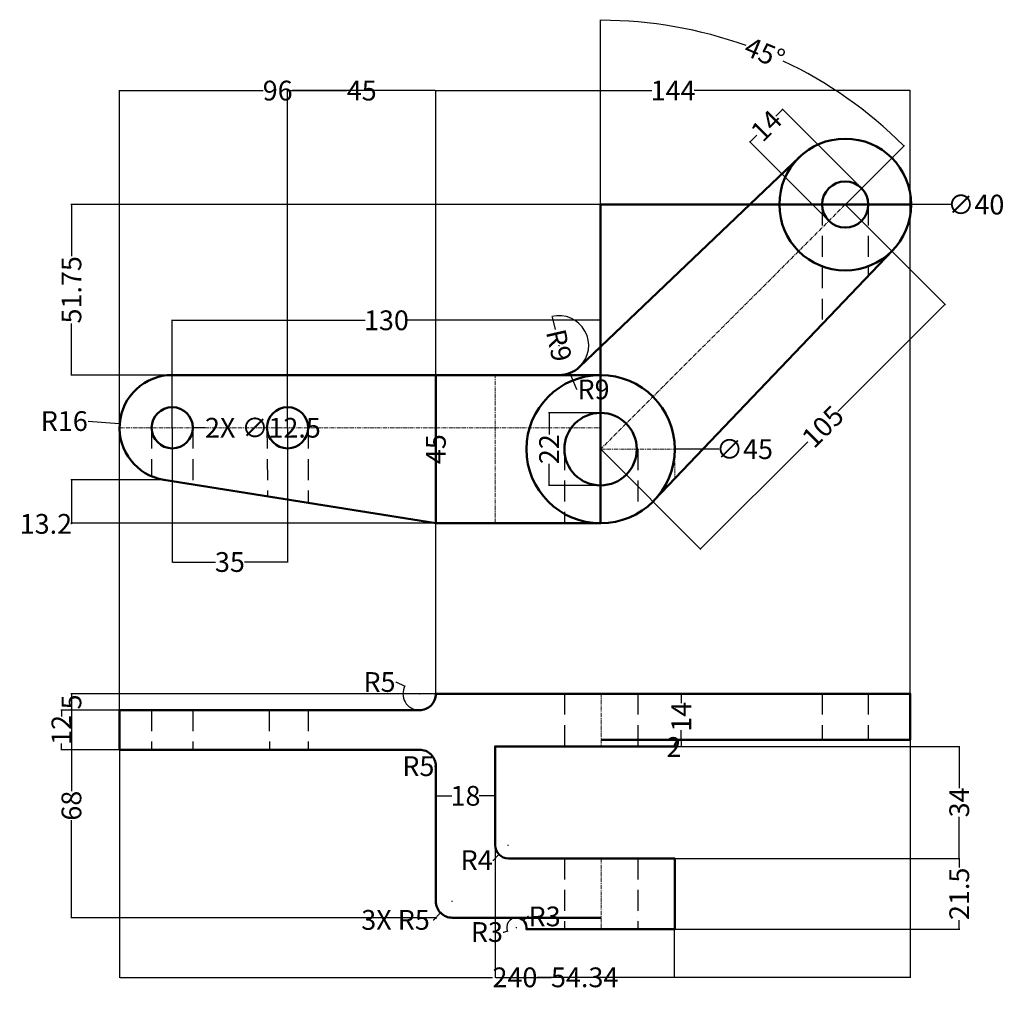
# Model space of a CAD drawing. Units: millimetres. Extents: x 160 to 459, y 38 to 332.
import ezdxf

# ---------------------------------------------------------------- set-up
doc = ezdxf.new("R2010")
doc.units = ezdxf.units.MM
doc.header["$MEASUREMENT"] = 0
doc.linetypes.add('CENTER', pattern=[2, 1.25, -0.25, 0.25, -0.25])
doc.linetypes.add('HIDDEN', pattern=[9.525, 6.35, -3.175])
for name, color, linetype, lineweight in [('M-CNTR', 4, 'CENTER', 18), ('M-DIMS', 2, 'Continuous', 25), ('M-HIDN', 6, 'HIDDEN', 25), ('M-OUTL', 7, 'Continuous', 50)]:
    doc.layers.add(name, color=color, linetype=linetype, lineweight=lineweight)
doc.styles.get("Standard").update_dxf_attribs({"font": 'arial.ttf'})
doc.dimstyles.get("Standard").update_dxf_attribs({"dimtxt": 6, "dimasz": 0.18, "dimexe": 0.18, "dimexo": 0.0625, "dimgap": 0.09, "dimtad": 0, "dimtoh": 1, "dimdec": 0, "dimzin": 0, "dimdsep": 46, "dimtxsty": 'Standard', "dimcen": 0.09, "dimadec": 0, "dimazin": 0, "dimtfac": 1, "dimtdec": 0, "dimtofl": 0, "dimtmove": 0, "dimatfit": 3, "dimfxl": 1, "dimtolj": 1, "dimtzin": 0, "dimarcsym": 0})

# ---------------------------------------------------------------- blocks, each defined once
blk = doc.blocks.new('*D1')
at = {"layer": 'Defpoints', "color": 0, "transparency": 16777216}
for p in [(401.36, 314.77), (336.26, 276.27), (410.51, 276.27), (336.26, 233.12), (336.26, 202.03)]:
    blk.add_point(p, dxfattribs=at)
at = {"layer": 'M-DIMS', "color": 0, "lineweight": -2, "transparency": 16777216}
for p, q in [((336.26, 276.34), (336.26, 332.4)), ((410.55, 276.32), (428.45, 294.21))]:
    blk.add_line(p, q, dxfattribs=at)
for start, end in [(70.1839, 89.9208), (45.0792, 64.8161)]:
    blk.add_arc((336.26, 202.03), 130.19, start, end, dxfattribs=at)
at = {"layer": 'M-DIMS', "color": 0, "transparency": 16777216}
for points in [[(336.44, 332.18), (336.44, 332.24), (336.26, 332.22)], [(428.21, 294.23), (428.17, 294.19), (428.32, 294.08)]]:
    blk.add_solid(points, dxfattribs=at)
at = {"layer": 'M-DIMS', "color": 0, "transparency": 16777216, "insert": (386.08, 322.31), "char_height": 6, "attachment_point": 5, "rotation": 337.5}
blk.add_mtext('\\A1;45°', dxfattribs=at)
blk = doc.blocks.new('*D2')
at = {"layer": 'Defpoints', "color": 0, "transparency": 16777216}
for p in [(410.51, 276.27), (440.81, 245.97), (336.26, 202.03)]:
    blk.add_point(p, dxfattribs=at)
at = {"layer": 'M-DIMS', "color": 0, "lineweight": -2, "transparency": 16777216}
for p, q in [((410.55, 276.23), (440.94, 245.85)), ((440.68, 245.85), (408.25, 213.42)), ((366.69, 171.85), (399.12, 204.28)), ((336.31, 201.98), (366.69, 171.6))]:
    blk.add_line(p, q, dxfattribs=at)
at = {"layer": 'M-DIMS', "color": 0, "transparency": 16777216}
for points in [[(440.66, 245.87), (440.7, 245.83), (440.81, 245.97)], [(366.67, 171.88), (366.71, 171.83), (366.56, 171.73)]]:
    blk.add_solid(points, dxfattribs=at)
at = {"layer": 'M-DIMS', "color": 0, "transparency": 16777216, "insert": (403.69, 208.85), "char_height": 6, "attachment_point": 5, "rotation": 45}
blk.add_mtext('\\A1;105', dxfattribs=at)
blk = doc.blocks.new('*D3')
at = {"layer": 'Defpoints', "color": 0, "transparency": 16777216}
for p in [(206.26, 241.14), (206.26, 208.53), (336.26, 208.53)]:
    blk.add_point(p, dxfattribs=at)
at = {"layer": 'M-DIMS', "color": 0, "lineweight": -2, "transparency": 16777216}
for p, q in [((206.26, 208.59), (206.26, 241.32)), ((206.44, 241.14), (264.84, 241.14)), ((336.08, 241.14), (277.69, 241.14)), ((336.26, 208.59), (336.26, 241.32))]:
    blk.add_line(p, q, dxfattribs=at)
at = {"layer": 'M-DIMS', "color": 0, "transparency": 16777216}
for points in [[(206.44, 241.17), (206.44, 241.11), (206.26, 241.14)], [(336.08, 241.17), (336.08, 241.11), (336.26, 241.14)]]:
    blk.add_solid(points, dxfattribs=at)
at = {"layer": 'M-DIMS', "color": 0, "transparency": 16777216, "insert": (271.26, 241.14), "char_height": 6, "attachment_point": 5}
blk.add_mtext('\\A1;130', dxfattribs=at)
blk = doc.blocks.new('*D4')
at = {"layer": 'Defpoints', "color": 0, "transparency": 16777216}
for p in [(286.26, 224.53), (286.26, 179.53), (286.26, 179.53)]:
    blk.add_point(p, dxfattribs=at)
at = {"layer": 'M-DIMS', "color": 0, "lineweight": -2, "transparency": 16777216}
for p, q in [((286.26, 224.35), (286.26, 206.56)), ((286.32, 224.53), (286.44, 224.53)), ((286.26, 179.71), (286.26, 197.5)), ((286.32, 179.53), (286.44, 179.53))]:
    blk.add_line(p, q, dxfattribs=at)
at = {"layer": 'M-DIMS', "color": 0, "transparency": 16777216}
for points in [[(286.23, 224.35), (286.29, 224.35), (286.26, 224.53)], [(286.23, 179.71), (286.29, 179.71), (286.26, 179.53)]]:
    blk.add_solid(points, dxfattribs=at)
at = {"layer": 'M-DIMS', "color": 0, "transparency": 16777216, "insert": (286.26, 202.03), "char_height": 6, "attachment_point": 5, "rotation": 90}
blk.add_mtext('\\A1;45', dxfattribs=at)
blk = doc.blocks.new('*D5')
at = {"layer": 'Defpoints', "color": 0, "transparency": 16777216}
for p in [(336.26, 213.03), (320.63, 191.03), (336.26, 191.03)]:
    blk.add_point(p, dxfattribs=at)
at = {"layer": 'M-DIMS', "color": 0, "lineweight": -2, "transparency": 16777216}
for p, q in [((336.2, 213.03), (320.45, 213.03)), ((320.63, 212.85), (320.63, 206.44)), ((320.63, 191.21), (320.63, 197.62)), ((336.2, 191.03), (320.45, 191.03))]:
    blk.add_line(p, q, dxfattribs=at)
at = {"layer": 'M-DIMS', "color": 0, "transparency": 16777216}
for points in [[(320.6, 212.85), (320.66, 212.85), (320.63, 213.03)], [(320.6, 191.21), (320.66, 191.21), (320.63, 191.03)]]:
    blk.add_solid(points, dxfattribs=at)
at = {"layer": 'M-DIMS', "color": 0, "transparency": 16777216, "insert": (320.63, 202.03), "char_height": 6, "attachment_point": 5, "rotation": 90}
blk.add_mtext('\\A1;22', dxfattribs=at)
blk = doc.blocks.new('*D6')
at = {"layer": 'Defpoints', "color": 0, "transparency": 16777216}
for p in [(206.26, 208.53), (241.26, 208.53), (241.26, 167.77)]:
    blk.add_point(p, dxfattribs=at)
at = {"layer": 'M-DIMS', "color": 0, "lineweight": -2, "transparency": 16777216}
for p, q in [((206.26, 208.47), (206.26, 167.59)), ((241.26, 208.47), (241.26, 167.59)), ((206.44, 167.77), (219.35, 167.77)), ((241.08, 167.77), (228.17, 167.77))]:
    blk.add_line(p, q, dxfattribs=at)
at = {"layer": 'M-DIMS', "color": 0, "transparency": 16777216}
for points in [[(206.44, 167.8), (206.44, 167.74), (206.26, 167.77)], [(241.08, 167.8), (241.08, 167.74), (241.26, 167.77)]]:
    blk.add_solid(points, dxfattribs=at)
at = {"layer": 'M-DIMS', "color": 0, "transparency": 16777216, "insert": (223.76, 167.77), "char_height": 6, "attachment_point": 5}
blk.add_mtext('\\A1;35', dxfattribs=at)
blk = doc.blocks.new('*D7')
at = {"layer": 'Defpoints', "color": 0, "transparency": 16777216}
for p in [(321.65, 242.3), (323.65, 233.53)]:
    blk.add_point(p, dxfattribs=at)
at = {"layer": 'M-DIMS', "color": 0, "lineweight": -2, "transparency": 16777216}
blk.add_line((322.55, 238.34), (321.69, 242.13), dxfattribs=at)
blk.add_arc((323.65, 233.53), 9, 314.0336, 104.0031, dxfattribs=at)
at = {"layer": 'M-DIMS', "color": 0, "transparency": 16777216}
blk.add_solid([(321.72, 242.13), (321.66, 242.12), (321.65, 242.3)], dxfattribs=at)
at = {"layer": 'M-DIMS', "color": 0, "transparency": 16777216, "insert": (323.65, 233.53), "char_height": 6, "attachment_point": 5, "rotation": 282.8571}
blk.add_mtext('\\A1;R9', dxfattribs=at)
blk = doc.blocks.new('*D8')
at = {"layer": 'Defpoints', "color": 0, "transparency": 16777216}
for p in [(391.51, 305.17), (415.46, 281.22), (405.56, 271.33)]:
    blk.add_point(p, dxfattribs=at)
at = {"layer": 'M-DIMS', "color": 0, "lineweight": -2, "transparency": 16777216}
for p, q in [((391.38, 305.05), (389.45, 303.12)), ((415.41, 281.27), (391.38, 305.3)), ((381.74, 295.4), (383.66, 297.33)), ((405.51, 271.37), (381.48, 295.4))]:
    blk.add_line(p, q, dxfattribs=at)
at = {"layer": 'M-DIMS', "color": 0, "transparency": 16777216}
for points in [[(391.36, 305.07), (391.4, 305.03), (391.51, 305.17)], [(381.71, 295.42), (381.76, 295.38), (381.61, 295.27)]]:
    blk.add_solid(points, dxfattribs=at)
at = {"layer": 'M-DIMS', "color": 0, "transparency": 16777216, "insert": (386.56, 300.22), "char_height": 6, "attachment_point": 5, "rotation": 45}
blk.add_mtext('\\A1;14', dxfattribs=at)
blk = doc.blocks.new('*D9')
at = {"layer": 'Defpoints', "color": 0, "transparency": 16777216}
for p in [(276.81, 130.07), (281.26, 127.8)]:
    blk.add_point(p, dxfattribs=at)
at = {"layer": 'M-DIMS', "color": 0, "lineweight": -2, "transparency": 16777216}
for p, q in [((274.11, 131.35), (274.29, 131.35)), ((274.29, 131.35), (276.65, 130.15)), ((281.17, 127.8), (281.35, 127.8)), ((281.26, 127.71), (281.26, 127.89))]:
    blk.add_line(p, q, dxfattribs=at)
blk.add_arc((281.26, 127.8), 5, 150.9688, 269.2838, dxfattribs=at)
at = {"layer": 'M-DIMS', "color": 0, "transparency": 16777216}
blk.add_solid([(276.66, 130.18), (276.63, 130.12), (276.81, 130.07)], dxfattribs=at)
at = {"layer": 'M-DIMS', "color": 0, "transparency": 16777216, "insert": (269.16, 131.35), "char_height": 6, "attachment_point": 5}
blk.add_mtext('\\A1;R5', dxfattribs=at)
blk = doc.blocks.new('*D10')
at = {"layer": 'Defpoints', "color": 0, "transparency": 16777216}
for p in [(358.26, 127.8), (358.26, 113.8), (360.76, 113.8)]:
    blk.add_point(p, dxfattribs=at)
at = {"layer": 'M-DIMS', "color": 0, "lineweight": -2, "transparency": 16777216}
for p, q in [((358.32, 127.8), (360.94, 127.8)), ((360.76, 127.62), (360.76, 124.89)), ((360.76, 113.98), (360.76, 116.71)), ((358.32, 113.8), (360.94, 113.8))]:
    blk.add_line(p, q, dxfattribs=at)
at = {"layer": 'M-DIMS', "color": 0, "transparency": 16777216}
for points in [[(360.73, 127.62), (360.79, 127.62), (360.76, 127.8)], [(360.73, 113.98), (360.79, 113.98), (360.76, 113.8)]]:
    blk.add_solid(points, dxfattribs=at)
at = {"layer": 'M-DIMS', "color": 0, "transparency": 16777216, "insert": (360.76, 120.8), "char_height": 6, "attachment_point": 5, "rotation": 90}
blk.add_mtext('\\A1;14', dxfattribs=at)
blk = doc.blocks.new('*D11')
at = {"layer": 'Defpoints', "color": 0, "transparency": 16777216}
for p in [(347.51, 113.8), (347.51, 111.8), (360.76, 111.8)]:
    blk.add_point(p, dxfattribs=at)
at = {"layer": 'M-DIMS', "color": 0, "lineweight": -2, "transparency": 16777216}
for p, q in [((347.57, 113.8), (360.94, 113.8)), ((360.76, 113.62), (360.76, 111.98)), ((347.57, 111.8), (360.94, 111.8)), ((360.76, 111.62), (360.58, 111.62)), ((360.76, 111.8), (360.76, 111.62))]:
    blk.add_line(p, q, dxfattribs=at)
at = {"layer": 'M-DIMS', "color": 0, "transparency": 16777216}
for points in [[(360.73, 113.62), (360.79, 113.62), (360.76, 113.8)], [(360.73, 111.98), (360.79, 111.98), (360.76, 111.8)]]:
    blk.add_solid(points, dxfattribs=at)
at = {"layer": 'M-DIMS', "color": 0, "transparency": 16777216, "insert": (358.51, 111.62), "char_height": 6, "attachment_point": 5}
blk.add_mtext('\\A1;2', dxfattribs=at)
blk = doc.blocks.new('*D12')
at = {"layer": 'Defpoints', "color": 0, "transparency": 16777216}
for p in [(310.76, 56.8), (307.93, 55.82)]:
    blk.add_point(p, dxfattribs=at)
at = {"layer": 'M-DIMS', "color": 0, "lineweight": -2, "transparency": 16777216}
for p, q in [((310.67, 56.8), (310.85, 56.8)), ((310.76, 56.71), (310.76, 56.89)), ((306.68, 55.45), (306.86, 55.45)), ((306.86, 55.45), (307.76, 55.76))]:
    blk.add_line(p, q, dxfattribs=at)
blk.add_arc((310.76, 56.8), 3, 91.1937, 202.5469, dxfattribs=at)
at = {"layer": 'M-DIMS', "color": 0, "transparency": 16777216}
blk.add_solid([(307.75, 55.79), (307.77, 55.73), (307.93, 55.82)], dxfattribs=at)
at = {"layer": 'M-DIMS', "color": 0, "transparency": 16777216, "insert": (301.76, 55.45), "char_height": 6, "attachment_point": 5}
blk.add_mtext('\\A1;R3', dxfattribs=at)
blk = doc.blocks.new('*D13')
at = {"layer": 'Defpoints', "color": 0, "transparency": 16777216}
for p in [(304.26, 96.8), (286.26, 85.3), (304.26, 85.3)]:
    blk.add_point(p, dxfattribs=at)
at = {"layer": 'M-DIMS', "color": 0, "lineweight": -2, "transparency": 16777216}
for p, q in [((286.26, 85.36), (286.26, 96.98)), ((286.44, 96.8), (291.15, 96.8)), ((304.08, 96.8), (299.37, 96.8)), ((304.26, 85.36), (304.26, 96.98))]:
    blk.add_line(p, q, dxfattribs=at)
at = {"layer": 'M-DIMS', "color": 0, "transparency": 16777216}
for points in [[(286.44, 96.83), (286.44, 96.77), (286.26, 96.8)], [(304.08, 96.83), (304.08, 96.77), (304.26, 96.8)]]:
    blk.add_solid(points, dxfattribs=at)
at = {"layer": 'M-DIMS', "color": 0, "transparency": 16777216, "insert": (295.26, 96.8), "char_height": 6, "attachment_point": 5}
blk.add_mtext('\\A1;18', dxfattribs=at)
blk = doc.blocks.new('*D14')
at = {"layer": 'Defpoints', "color": 0, "transparency": 16777216}
for p in [(281.26, 105.8), (286.26, 105.8)]:
    blk.add_point(p, dxfattribs=at)
at = {"layer": 'M-DIMS', "color": 0, "lineweight": -2, "transparency": 16777216}
blk.add_line((285.9, 105.8), (286.08, 105.8), dxfattribs=at)
at = {"layer": 'M-DIMS', "color": 0, "transparency": 16777216}
blk.add_solid([(286.08, 105.83), (286.08, 105.77), (286.26, 105.8)], dxfattribs=at)
at = {"layer": 'M-DIMS', "color": 0, "transparency": 16777216, "insert": (280.95, 105.8), "char_height": 6, "attachment_point": 5}
blk.add_mtext('\\A1;R5', dxfattribs=at)
blk = doc.blocks.new('*D15')
at = {"layer": 'Defpoints', "color": 0, "transparency": 16777216}
for p in [(190.26, 122.8), (172.62, 110.8), (190.26, 110.8)]:
    blk.add_point(p, dxfattribs=at)
at = {"layer": 'M-DIMS', "color": 0, "lineweight": -2, "transparency": 16777216}
for p, q in [((190.2, 122.8), (172.44, 122.8)), ((172.62, 122.62), (172.62, 120.87)), ((190.2, 110.8), (172.44, 110.8)), ((172.62, 110.98), (172.62, 112.72))]:
    blk.add_line(p, q, dxfattribs=at)
at = {"layer": 'M-DIMS', "color": 0, "transparency": 16777216}
for points in [[(172.59, 122.62), (172.65, 122.62), (172.62, 122.8)], [(172.59, 110.98), (172.65, 110.98), (172.62, 110.8)]]:
    blk.add_solid(points, dxfattribs=at)
at = {"layer": 'M-DIMS', "color": 0, "transparency": 16777216, "insert": (172.62, 116.8), "char_height": 6, "attachment_point": 5, "rotation": 90}
blk.add_mtext('\\A1;12', dxfattribs=at)
blk = doc.blocks.new('*D16')
at = {"layer": 'Defpoints', "color": 0, "transparency": 16777216}
for p in [(286.26, 310.87), (286.26, 224.53), (241.26, 208.53)]:
    blk.add_point(p, dxfattribs=at)
at = {"layer": 'M-DIMS', "color": 0, "lineweight": -2, "transparency": 16777216}
for p, q in [((241.26, 208.59), (241.26, 311.05)), ((241.44, 310.87), (259.23, 310.87)), ((286.08, 310.87), (268.29, 310.87)), ((286.26, 224.59), (286.26, 311.05))]:
    blk.add_line(p, q, dxfattribs=at)
at = {"layer": 'M-DIMS', "color": 0, "transparency": 16777216}
for points in [[(241.44, 310.9), (241.44, 310.84), (241.26, 310.87)], [(286.08, 310.9), (286.08, 310.84), (286.26, 310.87)]]:
    blk.add_solid(points, dxfattribs=at)
at = {"layer": 'M-DIMS', "color": 0, "transparency": 16777216, "insert": (263.76, 310.87), "char_height": 6, "attachment_point": 5}
blk.add_mtext('\\A1;45', dxfattribs=at)
blk = doc.blocks.new('*D17')
at = {"layer": 'Defpoints', "color": 0, "transparency": 16777216}
for p in [(336.26, 276.27), (175.66, 224.53), (336.26, 224.53)]:
    blk.add_point(p, dxfattribs=at)
at = {"layer": 'M-DIMS', "color": 0, "lineweight": -2, "transparency": 16777216}
for p, q in [((336.2, 276.27), (175.48, 276.27)), ((175.66, 276.09), (175.66, 260.64)), ((175.66, 224.71), (175.66, 240.17)), ((336.2, 224.53), (175.48, 224.53))]:
    blk.add_line(p, q, dxfattribs=at)
at = {"layer": 'M-DIMS', "color": 0, "transparency": 16777216}
for points in [[(175.63, 276.09), (175.69, 276.09), (175.66, 276.27)], [(175.63, 224.71), (175.69, 224.71), (175.66, 224.53)]]:
    blk.add_solid(points, dxfattribs=at)
at = {"layer": 'M-DIMS', "color": 0, "transparency": 16777216, "insert": (175.66, 250.4), "char_height": 6, "attachment_point": 5, "rotation": 90}
blk.add_mtext('\\A1;51.75', dxfattribs=at)
blk = doc.blocks.new('*D18')
at = {"layer": 'Defpoints', "color": 0, "transparency": 16777216}
for p in [(203.73, 192.73), (175.66, 179.53), (286.26, 179.53)]:
    blk.add_point(p, dxfattribs=at)
at = {"layer": 'M-DIMS', "color": 0, "lineweight": -2, "transparency": 16777216}
for p, q in [((203.67, 192.73), (175.48, 192.73)), ((175.66, 192.55), (175.66, 179.71)), ((286.2, 179.53), (175.48, 179.53)), ((175.66, 179.35), (175.48, 179.35)), ((175.66, 179.53), (175.66, 179.35))]:
    blk.add_line(p, q, dxfattribs=at)
at = {"layer": 'M-DIMS', "color": 0, "transparency": 16777216}
for points in [[(175.63, 192.55), (175.69, 192.55), (175.66, 192.73)], [(175.63, 179.71), (175.69, 179.71), (175.66, 179.53)]]:
    blk.add_solid(points, dxfattribs=at)
at = {"layer": 'M-DIMS', "color": 0, "transparency": 16777216, "insert": (167.91, 179.35), "char_height": 6, "attachment_point": 5}
blk.add_mtext('\\A1;13.2', dxfattribs=at)
blk = doc.blocks.new('*D19')
at = {"layer": 'Defpoints', "color": 0, "transparency": 16777216}
for p in [(430.26, 127.8), (190.26, 110.8), (430.26, 41.7)]:
    blk.add_point(p, dxfattribs=at)
at = {"layer": 'M-DIMS', "color": 0, "lineweight": -2, "transparency": 16777216}
for p, q in [((430.26, 127.74), (430.26, 41.52)), ((190.26, 110.74), (190.26, 41.52)), ((190.44, 41.7), (303.5, 41.7)), ((430.08, 41.7), (317.02, 41.7))]:
    blk.add_line(p, q, dxfattribs=at)
at = {"layer": 'M-DIMS', "color": 0, "transparency": 16777216}
for points in [[(190.44, 41.73), (190.44, 41.67), (190.26, 41.7)], [(430.08, 41.73), (430.08, 41.67), (430.26, 41.7)]]:
    blk.add_solid(points, dxfattribs=at)
at = {"layer": 'M-DIMS', "color": 0, "transparency": 16777216, "insert": (310.26, 41.7), "char_height": 6, "attachment_point": 5}
blk.add_mtext('\\A1;240', dxfattribs=at)
blk = doc.blocks.new('*D20')
at = {"layer": 'Defpoints', "color": 0, "transparency": 16777216}
for p in [(286.26, 310.87), (286.26, 127.8), (190.26, 122.8)]:
    blk.add_point(p, dxfattribs=at)
at = {"layer": 'M-DIMS', "color": 0, "lineweight": -2, "transparency": 16777216}
for p, q in [((190.26, 122.86), (190.26, 311.05)), ((190.44, 310.87), (233.88, 310.87)), ((286.08, 310.87), (242.65, 310.87)), ((286.26, 127.86), (286.26, 311.05))]:
    blk.add_line(p, q, dxfattribs=at)
at = {"layer": 'M-DIMS', "color": 0, "transparency": 16777216}
for points in [[(190.44, 310.9), (190.44, 310.84), (190.26, 310.87)], [(286.08, 310.9), (286.08, 310.84), (286.26, 310.87)]]:
    blk.add_solid(points, dxfattribs=at)
at = {"layer": 'M-DIMS', "color": 0, "transparency": 16777216, "insert": (238.26, 310.87), "char_height": 6, "attachment_point": 5}
blk.add_mtext('\\A1;96', dxfattribs=at)
blk = doc.blocks.new('*D21')
at = {"layer": 'Defpoints', "color": 0, "transparency": 16777216}
for p in [(430.26, 310.87), (286.26, 127.8), (430.26, 127.8)]:
    blk.add_point(p, dxfattribs=at)
at = {"layer": 'M-DIMS', "color": 0, "lineweight": -2, "transparency": 16777216}
for p, q in [((286.26, 127.86), (286.26, 311.05)), ((286.44, 310.87), (351.84, 310.87)), ((430.08, 310.87), (364.69, 310.87)), ((430.26, 127.86), (430.26, 311.05))]:
    blk.add_line(p, q, dxfattribs=at)
at = {"layer": 'M-DIMS', "color": 0, "transparency": 16777216}
for points in [[(286.44, 310.9), (286.44, 310.84), (286.26, 310.87)], [(430.08, 310.9), (430.08, 310.84), (430.26, 310.87)]]:
    blk.add_solid(points, dxfattribs=at)
at = {"layer": 'M-DIMS', "color": 0, "transparency": 16777216, "insert": (358.26, 310.87), "char_height": 6, "attachment_point": 5}
blk.add_mtext('\\A1;144', dxfattribs=at)
blk = doc.blocks.new('*D22')
at = {"layer": 'Defpoints', "color": 0, "transparency": 16777216}
for p in [(175.66, 127.8), (286.26, 127.8), (286.26, 59.8)]:
    blk.add_point(p, dxfattribs=at)
at = {"layer": 'M-DIMS', "color": 0, "lineweight": -2, "transparency": 16777216}
for p, q in [((286.2, 127.8), (175.48, 127.8)), ((175.66, 127.62), (175.66, 98.21)), ((175.66, 59.98), (175.66, 89.39)), ((286.2, 59.8), (175.48, 59.8))]:
    blk.add_line(p, q, dxfattribs=at)
at = {"layer": 'M-DIMS', "color": 0, "transparency": 16777216}
for points in [[(175.63, 127.62), (175.69, 127.62), (175.66, 127.8)], [(175.63, 59.98), (175.69, 59.98), (175.66, 59.8)]]:
    blk.add_solid(points, dxfattribs=at)
at = {"layer": 'M-DIMS', "color": 0, "transparency": 16777216, "insert": (175.66, 93.8), "char_height": 6, "attachment_point": 5, "rotation": 90}
blk.add_mtext('\\A1;68', dxfattribs=at)
blk = doc.blocks.new('*D23')
at = {"layer": 'Defpoints', "color": 0, "transparency": 16777216}
for p in [(175.66, 127.8), (286.26, 127.8), (190.26, 122.8)]:
    blk.add_point(p, dxfattribs=at)
at = {"layer": 'M-DIMS', "color": 0, "lineweight": -2, "transparency": 16777216}
for p, q in [((286.2, 127.8), (175.48, 127.8)), ((175.66, 127.62), (175.66, 127.38)), ((190.2, 122.8), (175.48, 122.8)), ((175.66, 122.98), (175.66, 123.22))]:
    blk.add_line(p, q, dxfattribs=at)
at = {"layer": 'M-DIMS', "color": 0, "transparency": 16777216}
for points in [[(175.63, 127.62), (175.69, 127.62), (175.66, 127.8)], [(175.63, 122.98), (175.69, 122.98), (175.66, 122.8)]]:
    blk.add_solid(points, dxfattribs=at)
at = {"layer": 'M-DIMS', "color": 0, "transparency": 16777216, "insert": (175.66, 125.3), "char_height": 6, "attachment_point": 5, "rotation": 90}
blk.add_mtext('\\A1;5', dxfattribs=at)
blk = doc.blocks.new('*D24')
at = {"layer": 'Defpoints', "color": 0, "transparency": 16777216}
for p in [(358.76, 111.8), (358.6, 77.8), (445.11, 77.8)]:
    blk.add_point(p, dxfattribs=at)
at = {"layer": 'M-DIMS', "color": 0, "lineweight": -2, "transparency": 16777216}
for p, q in [((358.82, 111.8), (445.29, 111.8)), ((445.11, 111.62), (445.11, 99.17)), ((445.11, 77.98), (445.11, 90.43)), ((358.67, 77.8), (445.29, 77.8))]:
    blk.add_line(p, q, dxfattribs=at)
at = {"layer": 'M-DIMS', "color": 0, "transparency": 16777216}
for points in [[(445.08, 111.62), (445.14, 111.62), (445.11, 111.8)], [(445.08, 77.98), (445.14, 77.98), (445.11, 77.8)]]:
    blk.add_solid(points, dxfattribs=at)
at = {"layer": 'M-DIMS', "color": 0, "transparency": 16777216, "insert": (445.11, 94.8), "char_height": 6, "attachment_point": 5, "rotation": 90}
blk.add_mtext('\\A1;34', dxfattribs=at)
blk = doc.blocks.new('*D25')
at = {"layer": 'Defpoints', "color": 0, "transparency": 16777216}
for p in [(358.6, 77.8), (358.76, 56.3), (445.11, 56.3)]:
    blk.add_point(p, dxfattribs=at)
at = {"layer": 'M-DIMS', "color": 0, "lineweight": -2, "transparency": 16777216}
for p, q in [((358.67, 77.8), (445.29, 77.8)), ((445.11, 77.62), (445.11, 75.01)), ((445.11, 56.48), (445.11, 59.09)), ((358.82, 56.3), (445.29, 56.3))]:
    blk.add_line(p, q, dxfattribs=at)
at = {"layer": 'M-DIMS', "color": 0, "transparency": 16777216}
for points in [[(445.08, 77.62), (445.14, 77.62), (445.11, 77.8)], [(445.08, 56.48), (445.14, 56.48), (445.11, 56.3)]]:
    blk.add_solid(points, dxfattribs=at)
at = {"layer": 'M-DIMS', "color": 0, "transparency": 16777216, "insert": (445.11, 67.05), "char_height": 6, "attachment_point": 5, "rotation": 90}
blk.add_mtext('\\A1;21.5', dxfattribs=at)
blk = doc.blocks.new('*D26')
at = {"layer": 'Defpoints', "color": 0, "transparency": 16777216}
for p in [(304.26, 111.8), (358.6, 77.8), (358.6, 41.7)]:
    blk.add_point(p, dxfattribs=at)
at = {"layer": 'M-DIMS', "color": 0, "lineweight": -2, "transparency": 16777216}
for p, q in [((304.26, 111.74), (304.26, 41.52)), ((358.6, 77.74), (358.6, 41.52)), ((304.44, 41.7), (321.23, 41.7)), ((358.42, 41.7), (341.63, 41.7))]:
    blk.add_line(p, q, dxfattribs=at)
at = {"layer": 'M-DIMS', "color": 0, "transparency": 16777216}
for points in [[(304.44, 41.73), (304.44, 41.67), (304.26, 41.7)], [(358.42, 41.73), (358.42, 41.67), (358.6, 41.7)]]:
    blk.add_solid(points, dxfattribs=at)
at = {"layer": 'M-DIMS', "color": 0, "transparency": 16777216, "insert": (331.43, 41.7), "char_height": 6, "attachment_point": 5}
blk.add_mtext('\\A1;54.34', dxfattribs=at)
blk = doc.blocks.new('*D27')
at = {"layer": 'Defpoints', "color": 0, "transparency": 16777216}
for p in [(313.76, 202.03), (358.76, 202.03)]:
    blk.add_point(p, dxfattribs=at)
at = {"layer": 'M-DIMS', "color": 0, "lineweight": -2, "transparency": 16777216}
for p, q in [((336.17, 202.03), (336.35, 202.03)), ((336.26, 201.94), (336.26, 202.12)), ((372.26, 202.03), (358.94, 202.03))]:
    blk.add_line(p, q, dxfattribs=at)
at = {"layer": 'M-DIMS', "color": 0, "transparency": 16777216}
blk.add_solid([(358.94, 202.06), (358.94, 202), (358.76, 202.03)], dxfattribs=at)
at = {"layer": 'M-DIMS', "color": 0, "transparency": 16777216, "insert": (379.94, 202.03), "char_height": 6, "attachment_point": 5}
blk.add_mtext('\\A1;∅45', dxfattribs=at)
blk = doc.blocks.new('*D28')
at = {"layer": 'Defpoints', "color": 0, "transparency": 16777216}
for p in [(390.51, 276.27), (430.51, 276.27)]:
    blk.add_point(p, dxfattribs=at)
at = {"layer": 'M-DIMS', "color": 0, "lineweight": -2, "transparency": 16777216}
for p, q in [((410.42, 276.27), (410.6, 276.27)), ((410.51, 276.18), (410.51, 276.36)), ((442.51, 276.27), (430.69, 276.27))]:
    blk.add_line(p, q, dxfattribs=at)
at = {"layer": 'M-DIMS', "color": 0, "transparency": 16777216}
blk.add_solid([(430.69, 276.31), (430.69, 276.25), (430.51, 276.27)], dxfattribs=at)
at = {"layer": 'M-DIMS', "color": 0, "transparency": 16777216, "insert": (450.15, 276.27), "char_height": 6, "attachment_point": 5}
blk.add_mtext('\\A1;∅40', dxfattribs=at)
blk = doc.blocks.new('*D29')
at = {"layer": 'Defpoints', "color": 0, "transparency": 16777216}
for p in [(190.31, 209.8), (206.26, 208.53)]:
    blk.add_point(p, dxfattribs=at)
at = {"layer": 'M-DIMS', "color": 0, "lineweight": -2, "transparency": 16777216}
for p, q in [((180.74, 210.56), (190.13, 209.81)), ((206.17, 208.53), (206.35, 208.53)), ((206.26, 208.44), (206.26, 208.62))]:
    blk.add_line(p, q, dxfattribs=at)
at = {"layer": 'M-DIMS', "color": 0, "transparency": 16777216}
blk.add_solid([(190.14, 209.84), (190.13, 209.78), (190.31, 209.8)], dxfattribs=at)
at = {"layer": 'M-DIMS', "color": 0, "transparency": 16777216, "insert": (173.49, 210.56), "char_height": 6, "attachment_point": 5}
blk.add_mtext('\\A1;R16', dxfattribs=at)
blk = doc.blocks.new('*D30')
at = {"layer": 'Defpoints', "color": 0, "transparency": 16777216}
for p in [(323.65, 233.53), (327, 225.17)]:
    blk.add_point(p, dxfattribs=at)
at = {"layer": 'M-DIMS', "color": 0, "lineweight": -2, "transparency": 16777216}
for p, q in [((323.56, 233.53), (323.74, 233.53)), ((323.65, 233.44), (323.65, 233.62)), ((329, 220.16), (327.06, 225.01)), ((329.18, 220.16), (329, 220.16))]:
    blk.add_line(p, q, dxfattribs=at)
at = {"layer": 'M-DIMS', "color": 0, "transparency": 16777216}
blk.add_solid([(327.09, 225.02), (327.04, 225), (327, 225.17)], dxfattribs=at)
at = {"layer": 'M-DIMS', "color": 0, "transparency": 16777216, "insert": (334.12, 220.16), "char_height": 6, "attachment_point": 5}
blk.add_mtext('\\A1;R9', dxfattribs=at)
blk = doc.blocks.new('*D31')
at = {"layer": 'Defpoints', "color": 0, "transparency": 16777216}
for p in [(200.01, 208.53), (212.51, 208.53)]:
    blk.add_point(p, dxfattribs=at)
at = {"layer": 'M-DIMS', "color": 0, "lineweight": -2, "transparency": 16777216}
for p, q in [((206.17, 208.53), (206.35, 208.53)), ((206.26, 208.44), (206.26, 208.62)), ((216.26, 208.53), (212.69, 208.53))]:
    blk.add_line(p, q, dxfattribs=at)
at = {"layer": 'M-DIMS', "color": 0, "transparency": 16777216}
blk.add_solid([(212.69, 208.56), (212.69, 208.5), (212.51, 208.53)], dxfattribs=at)
at = {"layer": 'M-DIMS', "color": 0, "transparency": 16777216, "insert": (233.77, 208.53), "char_height": 6, "attachment_point": 5}
blk.add_mtext('\\A1;2X ∅12.5', dxfattribs=at)
blk = doc.blocks.new('*D32')
at = {"layer": 'Defpoints', "color": 0, "transparency": 16777216}
for p in [(291.26, 64.8), (287.73, 61.26)]:
    blk.add_point(p, dxfattribs=at)
at = {"layer": 'M-DIMS', "color": 0, "lineweight": -2, "transparency": 16777216}
for p, q in [((291.17, 64.8), (291.35, 64.8)), ((291.26, 64.71), (291.26, 64.89)), ((285.61, 59.14), (287.6, 61.14)), ((285.43, 59.14), (285.61, 59.14))]:
    blk.add_line(p, q, dxfattribs=at)
at = {"layer": 'M-DIMS', "color": 0, "transparency": 16777216}
blk.add_solid([(287.58, 61.16), (287.62, 61.12), (287.73, 61.26)], dxfattribs=at)
at = {"layer": 'M-DIMS', "color": 0, "transparency": 16777216, "insert": (274.03, 59.14), "char_height": 6, "attachment_point": 5}
blk.add_mtext('\\A1;3X R5', dxfattribs=at)
blk = doc.blocks.new('*D33')
at = {"layer": 'Defpoints', "color": 0, "transparency": 16777216}
for p in [(308.26, 81.8), (305.43, 78.97)]:
    blk.add_point(p, dxfattribs=at)
at = {"layer": 'M-DIMS', "color": 0, "lineweight": -2, "transparency": 16777216}
for p, q in [((308.17, 81.8), (308.35, 81.8)), ((308.26, 81.71), (308.26, 81.89)), ((303.74, 77.27), (305.31, 78.84)), ((303.56, 77.27), (303.74, 77.27))]:
    blk.add_line(p, q, dxfattribs=at)
at = {"layer": 'M-DIMS', "color": 0, "transparency": 16777216}
blk.add_solid([(305.29, 78.86), (305.33, 78.82), (305.43, 78.97)], dxfattribs=at)
at = {"layer": 'M-DIMS', "color": 0, "transparency": 16777216, "insert": (298.64, 77.27), "char_height": 6, "attachment_point": 5}
blk.add_mtext('\\A1;R4', dxfattribs=at)
blk = doc.blocks.new('*D34')
at = {"layer": 'Defpoints', "color": 0, "transparency": 16777216}
for p in [(310.76, 56.8), (312.88, 58.92)]:
    blk.add_point(p, dxfattribs=at)
at = {"layer": 'M-DIMS', "color": 0, "lineweight": -2, "transparency": 16777216}
for p, q in [((314.16, 60.19), (313.01, 59.05)), ((314.34, 60.19), (314.16, 60.19)), ((310.67, 56.8), (310.85, 56.8)), ((310.76, 56.71), (310.76, 56.89))]:
    blk.add_line(p, q, dxfattribs=at)
at = {"layer": 'M-DIMS', "color": 0, "transparency": 16777216}
blk.add_solid([(312.99, 59.07), (313.03, 59.03), (312.88, 58.92)], dxfattribs=at)
at = {"layer": 'M-DIMS', "color": 0, "transparency": 16777216, "insert": (319.26, 60.19), "char_height": 6, "attachment_point": 5}
blk.add_mtext('\\A1;R3', dxfattribs=at)

msp = doc.modelspace()

# ---------------------------------------------------------------- linework, layer by layer
at = {"layer": 'M-CNTR'}
for p, q in [((304.262, 179.529), (304.262, 224.529)), ((190.262, 208.529), (336.262, 208.529)), ((336.387, 127.919), (336.387, 111.799)), ((336.387, 77.799), (336.387, 56.299)), ((347.512, 59.799), (347.512, 59.799))]:
    msp.add_line(p, q, dxfattribs=at)
msp.add_lwpolyline([(410.508, 276.275), (336.262, 202.029), (358.762, 202.029), (358.762, 193.021)], dxfattribs=at)
at = {"layer": 'M-HIDN'}
for p, q in [((403.508, 276.275), (403.508, 239.951)), ((417.508, 276.275), (417.508, 254.634)), ((200.012, 208.529), (200.012, 193.8)), ((212.512, 208.529), (212.512, 191.325)), ((235.012, 208.529), (235.172, 187.701)), ((247.512, 208.529), (247.512, 185.727)), ((325.262, 202.029), (325.262, 179.529)), ((347.512, 202.029), (347.512, 182.543)), ((325.262, 127.799), (325.262, 111.799)), ((347.512, 127.799), (347.512, 111.799)), ((403.508, 127.799), (403.508, 113.799)), ((417.508, 127.799), (417.508, 113.799)), ((200.012, 122.799), (200.012, 110.799)), ((212.512, 122.799), (212.512, 110.799)), ((235.67, 122.799), (235.762, 110.799)), ((247.512, 122.799), (247.512, 110.799)), ((325.262, 77.799), (325.262, 56.299)), ((347.512, 77.799), (347.512, 56.299))]:
    msp.add_line(p, q, dxfattribs=at)
at = {"layer": 'M-OUTL'}
for p, q in [((424.983, 262.473), (352.546, 186.502)), ((286.262, 224.529), (286.262, 179.529)), ((286.262, 127.799), (286.262, 127.799)), ((286.492, 59.799), (286.262, 59.799))]:
    msp.add_line(p, q, dxfattribs=at)
for points in [[(323.652, 224.529, 0.1927311), (329.862, 227.015), (396.707, 290.75)], [(336.262, 224.529), (336.262, 179.529), (286.262, 179.529), (203.735, 192.729, -0.9236794), (206.262, 224.529), (336.262, 224.529), (336.262, 233.117), (336.262, 276.275), (430.508, 276.275), (430.508, 276.209)], [(310.762, 59.799), (291.262, 59.799, -0.4142136), (286.262, 64.799), (286.262, 105.799, 0.4142136), (281.262, 110.799), (190.262, 110.799), (190.262, 122.799), (281.262, 122.799, 0.4142136), (286.262, 127.799), (430.262, 127.799), (430.262, 113.799), (360.762, 113.799), (336.387, 113.799)], [(360.762, 113.799, 0.4142136), (358.762, 111.799), (358.762, 111.799), (304.262, 111.799), (304.262, 81.799, 0.4142136), (308.262, 77.799), (358.605, 77.799), (358.762, 77.799)], [(358.762, 56.299), (358.762, 77.799), (358.762, 56.299), (313.762, 56.299), (313.762, 56.799, 0.4142136), (310.762, 59.799), (336.387, 59.799)]]:
    msp.add_lwpolyline(points, format="xyb", dxfattribs=at)
for centre, radius in [((410.508, 276.275), 20), ((410.508, 276.275), 7), ((336.262, 202.029), 22.5), ((206.262, 208.529), 6.25), ((241.262, 208.529), 6.25), ((336.262, 202.029), 11)]:
    msp.add_circle(centre, radius, dxfattribs=at)

# ---------------------------------------------------------------- dimensions: what is measured, and where the dimension line sits
at = {"layer": 'M-DIMS'}
dim = msp.add_angular_dim_2l(base=(401.355, 314.773), line1=((336.262, 233.117), (336.262, 276.275)), line2=((410.508, 276.275), (336.262, 202.029)), dimstyle='Standard', override={"dimclrd": 0, "dimclre": 0, "dimclrt": 0}, dxfattribs=at)
dim.commit()
dim.dimension.update_dxf_attribs({"geometry": '*D1', "text_midpoint": (386.082, 322.305)})
for base, p1, p2, override, picture, middle in [((286.262, 310.875), (190.262, 122.799), (286.262, 127.799), {"dimdec": 0, "dimlfac": 1, "dimrnd": 0, "dimzin": 0, "dimdsep": 46, "dimlunit": 2}, '*D20', (238.262, 310.875)), ((286.262, 310.875), (241.262, 208.529), (286.262, 224.529), {"dimdec": 0, "dimlfac": 1, "dimrnd": 0, "dimzin": 0, "dimdsep": 46, "dimlunit": 2}, '*D16', (263.762, 310.875)), ((430.262, 310.875), (286.262, 127.799), (430.262, 127.799), {"dimdec": 0, "dimlfac": 1, "dimrnd": 0, "dimzin": 0, "dimdsep": 46, "dimlunit": 2}, '*D21', (358.262, 310.875)), ((241.262, 167.774), (206.262, 208.529), (241.262, 208.529), {"dimclrd": 0, "dimclre": 0, "dimclrt": 0}, '*D6', (223.762, 167.774)), ((430.262, 41.699), (190.262, 110.799), (430.262, 127.799), {"dimdec": 0, "dimlfac": 1, "dimrnd": 0, "dimzin": 0, "dimdsep": 46, "dimlunit": 2}, '*D19', (310.262, 41.699)), ((358.605, 41.699), (304.262, 111.799), (358.605, 77.799), {"dimdec": 2, "dimlfac": 1, "dimrnd": 0, "dimzin": 0, "dimdsep": 46, "dimlunit": 2}, '*D26', (331.433, 41.699)), ((304.262, 96.799), (286.262, 85.299), (304.262, 85.299), {"dimclrd": 0, "dimclre": 0, "dimclrt": 0}, '*D13', (295.262, 96.799))]:
    dim = msp.add_linear_dim(base=base, p1=p1, p2=p2, dimstyle='Standard', override=override, dxfattribs=at)
    dim.commit()
    dim.dimension.update_dxf_attribs({"geometry": picture, "text_midpoint": middle})
for p1, p2, distance, picture, middle in [((405.559, 271.325), (415.458, 281.225), 33.87, '*D8', (386.559, 300.225)), ((336.262, 202.029), (410.508, 276.275), -42.852, '*D2', (403.686, 208.851)), ((336.262, 208.529), (206.262, 208.529), -32.612, '*D3', (271.262, 241.14))]:
    dim = msp.add_aligned_dim(p1=p1, p2=p2, distance=distance, dimstyle='Standard', override={"dimclrd": 0, "dimclre": 0, "dimclrt": 0}, dxfattribs=at)
    dim.commit()
    dim.dimension.update_dxf_attribs({"geometry": picture, "text_midpoint": middle})
for p1, p2, picture, middle in [((390.508, 276.275), (430.508, 276.275), '*D28', (442.508, 276.275)), ((313.762, 202.028), (358.762, 202.029), '*D27', (372.262, 202.029))]:
    dim = msp.add_diameter_dim_2p(p1=p1, p2=p2, dimstyle='Standard', override={"dimdec": 0, "dimlfac": 1, "dimrnd": 0, "dimzin": 0, "dimdsep": 46, "dimlunit": 2}, dxfattribs=at)
    dim.commit()
    dim.dimension.update_dxf_attribs({"geometry": picture, "text_midpoint": middle, "dimtype": 163})
for base, p1, p2, override, picture, middle in [((175.662, 224.529), (336.262, 276.275), (336.262, 224.529), {"dimdec": 2, "dimlfac": 1, "dimrnd": 0, "dimzin": 0, "dimdsep": 46, "dimlunit": 2}, '*D17', (175.662, 250.402)), ((286.262, 179.529), (286.262, 224.529), (286.262, 179.529), {"dimclrd": 0, "dimclre": 0, "dimclrt": 0}, '*D4', (286.262, 202.029)), ((320.63, 191.029), (336.262, 213.029), (336.262, 191.029), {"dimclrd": 0, "dimclre": 0, "dimclrt": 0}, '*D5', (320.63, 202.029)), ((175.662, 179.529), (203.735, 192.729), (286.262, 179.529), {"dimdec": 1, "dimlfac": 1, "dimrnd": 0, "dimzin": 0, "dimdsep": 46, "dimlunit": 2}, '*D18', (167.913, 179.349)), ((175.662, 127.799), (286.262, 59.799), (286.262, 127.799), {"dimdec": 0, "dimlfac": 1, "dimrnd": 0, "dimzin": 0, "dimdsep": 46, "dimlunit": 2}, '*D22', (175.662, 93.799)), ((175.662, 127.799), (190.262, 122.799), (286.262, 127.799), {"dimdec": 0, "dimlfac": 1, "dimrnd": 0, "dimzin": 0, "dimdsep": 46, "dimlunit": 2}, '*D23', (175.662, 125.299)), ((360.762, 113.799), (358.262, 127.799), (358.262, 113.799), {"dimclrd": 0, "dimclre": 0, "dimclrt": 0}, '*D10', (360.762, 120.799)), ((172.625, 110.799), (190.262, 122.799), (190.262, 110.799), {"dimclrd": 0, "dimclre": 0, "dimclrt": 0}, '*D15', (172.625, 116.799)), ((360.762, 111.799), (347.512, 113.799), (347.512, 111.799), {"dimclrd": 0, "dimclre": 0, "dimclrt": 0}, '*D11', (358.505, 111.619)), ((445.108, 77.799), (358.762, 111.799), (358.605, 77.799), {"dimdec": 0, "dimlfac": 1, "dimrnd": 0, "dimzin": 0, "dimdsep": 46, "dimlunit": 2}, '*D24', (445.108, 94.799)), ((445.108, 56.299), (358.605, 77.799), (358.762, 56.299), {"dimdec": 1, "dimlfac": 1, "dimrnd": 0, "dimzin": 0, "dimdsep": 46, "dimlunit": 2}, '*D25', (445.108, 67.049))]:
    dim = msp.add_linear_dim(base=base, p1=p1, p2=p2, angle=90, dimstyle='Standard', override=override, dxfattribs=at)
    dim.commit()
    dim.dimension.update_dxf_attribs({"geometry": picture, "text_midpoint": middle})
for center, mpoint, override, picture, middle in [((323.652, 233.529), (321.649, 242.303), {"dimclrd": 0, "dimclre": 0, "dimclrt": 0}, '*D7', (323.652, 233.529)), ((323.652, 233.529), (326.997, 225.173), {"dimdec": 0, "dimlfac": 1, "dimrnd": 0, "dimzin": 0, "dimdsep": 46, "dimlunit": 2}, '*D30', (334.118, 220.16)), ((206.262, 208.529), (190.312, 209.796), {"dimdec": 0, "dimlfac": 1, "dimrnd": 0, "dimzin": 0, "dimdsep": 46, "dimlunit": 2}, '*D29', (180.743, 210.556)), ((281.262, 127.799), (276.806, 130.067), {"dimclrd": 0, "dimclre": 0, "dimclrt": 0}, '*D9', (269.16, 131.347)), ((281.262, 105.799), (286.262, 105.799), {"dimclrd": 0, "dimclre": 0, "dimclrt": 0}, '*D14', (280.952, 105.799)), ((308.262, 81.799), (305.434, 78.971), {"dimdec": 0, "dimlfac": 1, "dimrnd": 0, "dimzin": 0, "dimdsep": 46, "dimlunit": 2}, '*D33', (298.641, 77.274)), ((310.762, 56.799), (312.884, 58.92), {"dimdec": 0, "dimlfac": 1, "dimrnd": 0, "dimzin": 0, "dimdsep": 46, "dimlunit": 2}, '*D34', (319.265, 60.192)), ((310.762, 56.799), (307.927, 55.817), {"dimclrd": 0, "dimclre": 0, "dimclrt": 0}, '*D12', (301.755, 55.448))]:
    dim = msp.add_radius_dim(center=center, mpoint=mpoint, dimstyle='Standard', override=override, dxfattribs=at)
    dim.commit()
    dim.dimension.update_dxf_attribs({"geometry": picture, "text_midpoint": middle, "dimtype": 164})
dim = msp.add_diameter_dim_2p(p1=(200.012, 208.528), p2=(212.512, 208.529), text='2X <>', dimstyle='Standard', override={"dimdec": 1, "dimlfac": 1, "dimrnd": 0, "dimzin": 0, "dimdsep": 46, "dimlunit": 2}, dxfattribs=at)
dim.commit()
dim.dimension.update_dxf_attribs({"geometry": '*D31', "text_midpoint": (216.262, 208.529), "dimtype": 163})
dim = msp.add_radius_dim(center=(291.262, 64.799), mpoint=(287.727, 61.264), text='3X <>', dimstyle='Standard', override={"dimdec": 0, "dimlfac": 1, "dimrnd": 0, "dimzin": 0, "dimdsep": 46, "dimlunit": 2}, dxfattribs=at)
dim.commit()
dim.dimension.update_dxf_attribs({"geometry": '*D32', "text_midpoint": (274.031, 59.142), "dimtype": 164})

doc.saveas('drawing.dxf')
